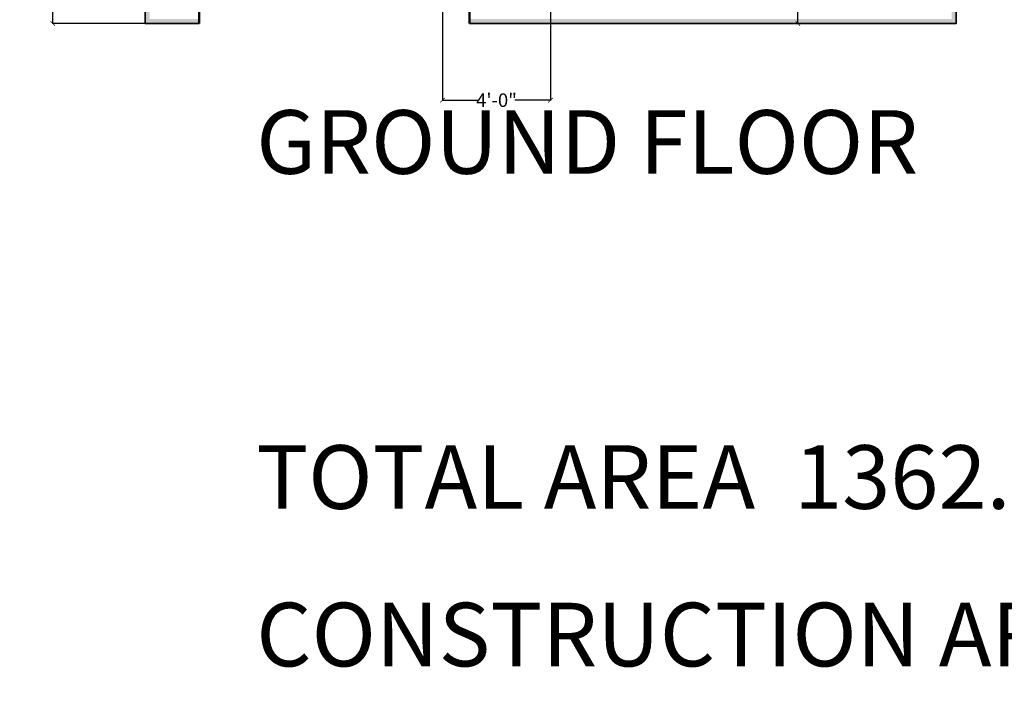
# Model space of a CAD drawing. Units: inches. Extents: x 528 to 2620, y -1066 to 798.
# Tile 1 of 41: x 528 to 966, y -83 to 211. Entities that reach past the tile are written whole.
import ezdxf

# ---------------------------------------------------------------- set-up
doc = ezdxf.new("R2010")
doc.units = ezdxf.units.IN
doc.header["$MEASUREMENT"] = 0
for name, color, linetype, lineweight in [('A-ANNO-DIMS', 2, 'Continuous', 18), ('A-ANNO-TEXT', 7, 'Continuous', 25), ('A-WALL', 7, 'Continuous', 50), ('A-WALL-PATT', 8, 'Continuous', 13), ('C-PROP', 5, 'Continuous', 35)]:
    doc.layers.add(name, color=color, linetype=linetype, lineweight=lineweight)
doc.styles.get("Standard").update_dxf_attribs({"font": 'arial.ttf'})
doc.dimstyles.get("Standard").update_dxf_attribs({"dimtxt": 6, "dimasz": 2, "dimexe": 0.18, "dimexo": 0.0625, "dimgap": 0.09, "dimtad": 0, "dimtih": 1, "dimtoh": 1, "dimdec": 1, "dimzin": 0, "dimdsep": 46, "dimlunit": 3, "dimtxsty": 'Standard', "dimblk": 'ARCHTICK', "dimcen": 0.09, "dimadec": 0, "dimazin": 0, "dimtfac": 1, "dimtdec": 1, "dimtofl": 0, "dimtmove": 0, "dimatfit": 3, "dimfxl": 1, "dimtolj": 1, "dimtzin": 0, "dimarcsym": 0})

# ---------------------------------------------------------------- blocks, each defined once
blk = doc.blocks.new('_ArchTick')
at = {"color": 0, "linetype": 'ByBlock', "const_width": 0.15}
blk.add_lwpolyline([(-0.5, -0.5), (0.5, 0.5)], dxfattribs=at)
blk = doc.blocks.new('*D12')
at = {"layer": 'A-ANNO-DIMS', "color": 0, "lineweight": -2, "transparency": 16777216}
for p, q in [((584, 753.92), (542.88, 753.92)), ((543.06, 753.92), (543.06, 484.58)), ((543.06, 208.92), (543.06, 478.27)), ((584, 208.92), (542.88, 208.92))]:
    blk.add_line(p, q, dxfattribs=at)
at = {"layer": 'Defpoints', "color": 0, "transparency": 16777216}
for p in [(584.06, 753.92), (543.06, 208.92), (584.06, 208.92)]:
    blk.add_point(p, dxfattribs=at)
at = {"layer": 'A-ANNO-DIMS', "color": 0, "lineweight": -2, "transparency": 16777216, "xscale": 2, "yscale": 2, "zscale": 2}
for p, rotation in [((543.06, 753.92), 90), ((543.06, 208.92), 270)]:
    blk.add_blockref('_ArchTick', p, dxfattribs=dict(at, rotation=rotation))
at = {"layer": 'A-ANNO-DIMS', "color": 0, "transparency": 16777216, "insert": (543.06, 481.42), "char_height": 6, "attachment_point": 5}
blk.add_mtext('\\A1;45\'-5.0"', dxfattribs=at)
blk = doc.blocks.new('*D15')
at = {"layer": 'A-ANNO-DIMS', "color": 0, "lineweight": -2, "transparency": 16777216}
for p, q in [((872.31, 268.92), (874.04, 268.92)), ((873.86, 268.92), (873.86, 242.06)), ((873.86, 208.92), (873.86, 235.78)), ((872.31, 208.92), (874.04, 208.92))]:
    blk.add_line(p, q, dxfattribs=at)
at = {"layer": 'Defpoints', "color": 0, "transparency": 16777216}
for p in [(872.24, 268.92), (872.24, 208.92), (873.86, 208.92)]:
    blk.add_point(p, dxfattribs=at)
at = {"layer": 'A-ANNO-DIMS', "color": 0, "lineweight": -2, "transparency": 16777216, "xscale": 2, "yscale": 2, "zscale": 2}
for p, rotation in [((873.86, 268.92), 90), ((873.86, 208.92), 270)]:
    blk.add_blockref('_ArchTick', p, dxfattribs=dict(at, rotation=rotation))
at = {"layer": 'A-ANNO-DIMS', "color": 0, "transparency": 16777216, "insert": (873.86, 238.92), "char_height": 6, "attachment_point": 5}
blk.add_mtext("\\A1;5'", dxfattribs=at)
blk = doc.blocks.new('*D57')
at = {"layer": 'A-ANNO-DIMS', "color": 0, "lineweight": -2, "transparency": 16777216}
for p, q in [((716.06, 391.36), (716.06, 174.74)), ((764.06, 391.36), (764.06, 174.74)), ((716.06, 174.92), (731.87, 174.92)), ((764.06, 174.92), (748.24, 174.92))]:
    blk.add_line(p, q, dxfattribs=at)
at = {"layer": 'Defpoints', "color": 0, "transparency": 16777216}
for p in [(716.06, 391.42), (764.06, 391.42), (764.06, 174.92)]:
    blk.add_point(p, dxfattribs=at)
at = {"layer": 'A-ANNO-DIMS', "color": 0, "lineweight": -2, "transparency": 16777216, "xscale": 2, "yscale": 2, "zscale": 2, "rotation": 180}
blk.add_blockref('_ArchTick', (716.06, 174.92), dxfattribs=at)
at = {"layer": 'A-ANNO-DIMS', "color": 0, "lineweight": -2, "transparency": 16777216, "xscale": 2, "yscale": 2, "zscale": 2}
blk.add_blockref('_ArchTick', (764.06, 174.92), dxfattribs=at)
at = {"layer": 'A-ANNO-DIMS', "color": 0, "transparency": 16777216, "insert": (740.06, 174.92), "char_height": 6, "attachment_point": 5}
blk.add_mtext('\\A1;4\'-0"', dxfattribs=at)

msp = doc.modelspace()

# ---------------------------------------------------------------- hatches: boundary and pattern name
at = {"layer": 'A-WALL-PATT', "transparency": 33554687}
h = msp.add_hatch(color=256, dxfattribs=at)
h.dxf.hatch_style = 1
h.paths.add_polyline_path([(944.06, 753.92), (584.06, 753.92), (584.06, 208.92), (608.06, 208.92), (608.06, 210.92), (586.06, 210.92), (586.06, 751.92), (942.06, 751.92), (942.06, 210.92), (728.06, 210.92), (728.06, 208.92), (944.06, 208.92)])

# ---------------------------------------------------------------- linework, layer by layer
at = {"layer": 'A-WALL'}
for p, q in [((608.06, 220.92), (608.06, 208.92)), ((728.06, 220.92), (728.06, 208.92))]:
    msp.add_line(p, q, dxfattribs=at)
at = {"layer": 'C-PROP'}
msp.add_lwpolyline([(728.06, 208.92), (944.06, 208.92), (944.06, 753.92), (584.06, 753.92), (584.06, 208.92), (608.06, 208.92)], dxfattribs=at)

# ---------------------------------------------------------------- texts
at = {"layer": 'A-ANNO-TEXT'}
for s, p in [('GROUND FLOOR', (633.4, 142.26)), ('TOTAL AREA  1362.500 SQUREFEET', (633.4, -6.41)), ('CONSTRUCTION AREA  772. 396 SQUREFEETS', (633.4, -76.3))]:
    msp.add_text(s, height=28.2129, dxfattribs=at).set_placement(p)

# ---------------------------------------------------------------- dimensions: what is measured, and where the dimension line sits
at = {"layer": 'A-ANNO-DIMS'}
for base, p1, p2, picture, middle in [((543.06, 208.92), (584.06, 753.92), (584.06, 208.92), '*D12', (543.06, 481.42)), ((873.86, 208.92), (872.24, 268.92), (872.24, 208.92), '*D15', (873.86, 238.92))]:
    dim = msp.add_linear_dim(base=base, p1=p1, p2=p2, angle=90, dimstyle='Standard', override={"dimclrd": 0, "dimclre": 0, "dimclrt": 0}, dxfattribs=at)
    dim.commit()
    dim.dimension.update_dxf_attribs({"geometry": picture, "text_midpoint": middle})
dim = msp.add_linear_dim(base=(764.06, 174.92), p1=(716.06, 391.42), p2=(764.06, 391.42), dimstyle='Standard', override={"dimdec": 1, "dimlfac": 1, "dimrnd": 0, "dimzin": 1, "dimdsep": 46, "dimlunit": 4, "dimfrac": 2}, dxfattribs=at)
dim.commit()
dim.dimension.update_dxf_attribs({"geometry": '*D57', "text_midpoint": (740.06, 174.92)})

doc.saveas('drawing.dxf')
